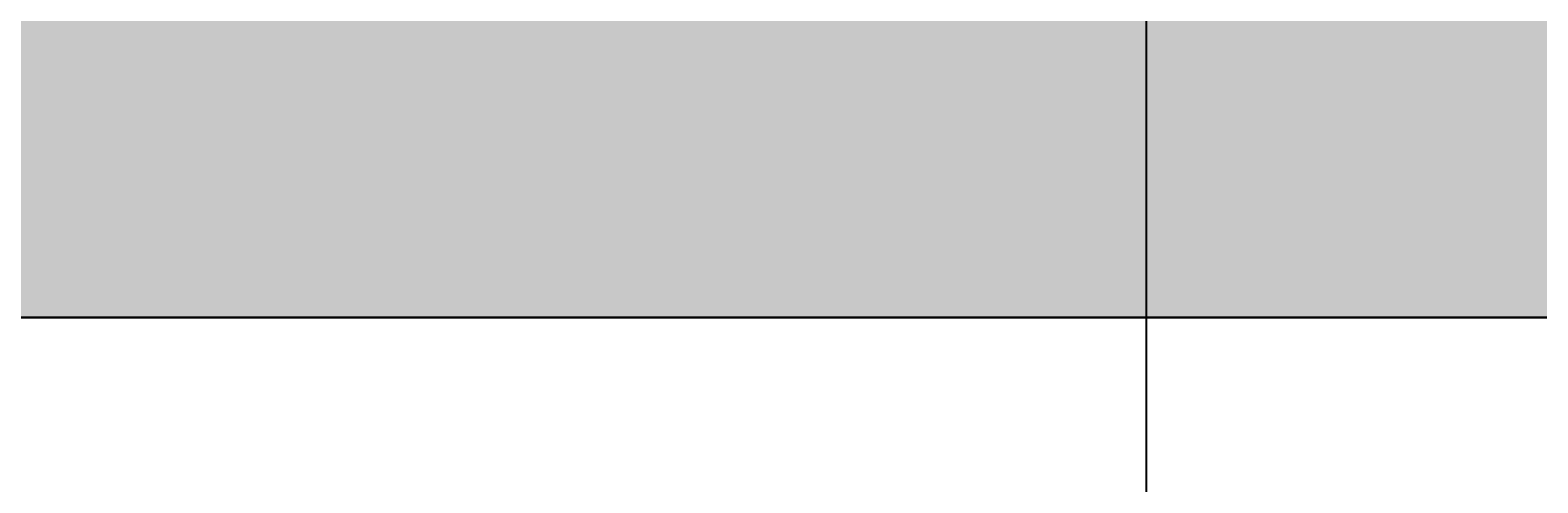
# Model space of a CAD drawing. Units: inches. Extents: x -301 to 715, y -607 to 364.
# Tile 16 of 141: x 18 to 59, y -486 to -474. Entities that reach past the tile are written whole.
import ezdxf

# ---------------------------------------------------------------- set-up
doc = ezdxf.new("R2010")
doc.units = ezdxf.units.IN
doc.header["$MEASUREMENT"] = 0
for name, color, linetype, lineweight in [('A-ANNO-DIMS', 2, 'Continuous', 18), ('A-GRND', 7, 'Continuous', 25), ('A-SECT-PATT', 8, 'Continuous', 13)]:
    doc.layers.add(name, color=color, linetype=linetype, lineweight=lineweight)
doc.styles.get("Standard").update_dxf_attribs({"font": 'arial.ttf'})
doc.dimstyles.get("Standard").update_dxf_attribs({"dimtxt": 0.18, "dimasz": 0.18, "dimexe": 0.18, "dimexo": 0.0625, "dimgap": 0.09, "dimtad": 0, "dimtih": 1, "dimtoh": 1, "dimdec": 1, "dimzin": 0, "dimdsep": 46, "dimlunit": 4, "dimtxsty": 'Standard', "dimcen": 0.09, "dimclrd": 3, "dimclre": 4, "dimclrt": 6, "dimadec": 0, "dimazin": 0, "dimtfac": 1, "dimtdec": 1, "dimtofl": 0, "dimtmove": 0, "dimatfit": 3, "dimfxl": 1, "dimtfill": 2, "dimtfillclr": 51, "dimtolj": 1, "dimtzin": 0, "dimarcsym": 0})

# ---------------------------------------------------------------- blocks, each defined once
blk = doc.blocks.new('*D176')
at = {"layer": 'A-ANNO-DIMS', "color": 4, "lineweight": -2, "transparency": 16777216}
for p, q in [((148.28, -324.477), (215.605, -324.477)), ((-15.22, -540.477), (215.605, -540.477))]:
    blk.add_line(p, q, dxfattribs=at)
at = {"layer": 'A-ANNO-DIMS', "color": 3, "lineweight": -2, "transparency": 16777216}
for p, q in [((215.425, -324.657), (215.425, -432.296)), ((215.425, -540.297), (215.425, -432.659))]:
    blk.add_line(p, q, dxfattribs=at)
at = {"layer": 'A-ANNO-DIMS', "color": 3, "transparency": 16777216}
for points in [[(215.395, -324.657), (215.455, -324.657), (215.425, -324.477)], [(215.395, -540.297), (215.455, -540.297), (215.425, -540.477)]]:
    blk.add_solid(points, dxfattribs=at)
at = {"layer": 'Defpoints', "color": 0, "transparency": 16777216}
for p in [(148.218, -324.477), (-15.282, -540.477), (215.425, -540.477)]:
    blk.add_point(p, dxfattribs=at)
at = {"layer": 'A-ANNO-DIMS', "color": 6, "transparency": 16777216, "insert": (215.425, -432.477), "char_height": 0.18, "attachment_point": 5, "bg_fill": 1, "box_fill_scale": 1.25, "bg_fill_color": 51, "bg_fill_transparency": 0}
blk.add_mtext('\\A1;18\'-0"', dxfattribs=at)
blk = doc.blocks.new('*D181')
at = {"layer": 'A-ANNO-DIMS', "color": 4, "lineweight": -2, "transparency": 16777216}
for p, q in [((48.468, -433.54), (48.468, -573.809)), ((12.718, -463.54), (12.718, -573.809))]:
    blk.add_line(p, q, dxfattribs=at)
at = {"layer": 'A-ANNO-DIMS', "color": 3, "lineweight": -2, "transparency": 16777216}
for p, q in [((12.898, -573.629), (30.264, -573.629)), ((48.288, -573.629), (30.922, -573.629))]:
    blk.add_line(p, q, dxfattribs=at)
at = {"layer": 'A-ANNO-DIMS', "color": 3, "transparency": 16777216}
for points in [[(12.898, -573.599), (12.898, -573.659), (12.718, -573.629)], [(48.288, -573.599), (48.288, -573.659), (48.468, -573.629)]]:
    blk.add_solid(points, dxfattribs=at)
at = {"layer": 'Defpoints', "color": 0, "transparency": 16777216}
for p in [(48.468, -433.477), (12.718, -463.477), (48.468, -573.629)]:
    blk.add_point(p, dxfattribs=at)
at = {"layer": 'A-ANNO-DIMS', "color": 6, "transparency": 16777216, "insert": (30.593, -573.629), "char_height": 0.18, "attachment_point": 5, "bg_fill": 1, "box_fill_scale": 1.25, "bg_fill_color": 51, "bg_fill_transparency": 0}
blk.add_mtext('\\A1;3\'-0"', dxfattribs=at)
blk = doc.blocks.new('*D190')
at = {"layer": 'A-ANNO-DIMS', "color": 4, "lineweight": -2, "transparency": 16777216}
for p, q in [((129.193, -481.477), (-266.112, -481.477)), ((124.193, -511.477), (-266.112, -511.477))]:
    blk.add_line(p, q, dxfattribs=at)
at = {"layer": 'A-ANNO-DIMS', "color": 3, "lineweight": -2, "transparency": 16777216}
for p, q in [((-265.932, -481.657), (-265.932, -496.296)), ((-265.932, -511.297), (-265.932, -496.659))]:
    blk.add_line(p, q, dxfattribs=at)
at = {"layer": 'A-ANNO-DIMS', "color": 3, "transparency": 16777216}
for points in [[(-265.962, -481.657), (-265.902, -481.657), (-265.932, -481.477)], [(-265.962, -511.297), (-265.902, -511.297), (-265.932, -511.477)]]:
    blk.add_solid(points, dxfattribs=at)
at = {"layer": 'Defpoints', "color": 0, "transparency": 16777216}
for p in [(129.255, -481.477), (-265.932, -511.477), (124.255, -511.477)]:
    blk.add_point(p, dxfattribs=at)
at = {"layer": 'A-ANNO-DIMS', "color": 6, "transparency": 16777216, "insert": (-265.932, -496.477), "char_height": 0.18, "attachment_point": 5, "bg_fill": 1, "box_fill_scale": 1.25, "bg_fill_color": 51, "bg_fill_transparency": 0}
blk.add_mtext('\\A1;2\'-6"', dxfattribs=at)
blk = doc.blocks.new('*D191')
at = {"layer": 'A-ANNO-DIMS', "color": 4, "lineweight": -2, "transparency": 16777216}
for p, q in [((129.193, -481.477), (-266.112, -481.477)), ((114.193, -540.477), (-266.112, -540.477))]:
    blk.add_line(p, q, dxfattribs=at)
at = {"layer": 'A-ANNO-DIMS', "color": 3, "lineweight": -2, "transparency": 16777216}
for p, q in [((-265.932, -481.657), (-265.932, -510.797)), ((-265.932, -540.297), (-265.932, -511.158))]:
    blk.add_line(p, q, dxfattribs=at)
at = {"layer": 'A-ANNO-DIMS', "color": 3, "transparency": 16777216}
for points in [[(-265.962, -481.657), (-265.902, -481.657), (-265.932, -481.477)], [(-265.962, -540.297), (-265.902, -540.297), (-265.932, -540.477)]]:
    blk.add_solid(points, dxfattribs=at)
at = {"layer": 'Defpoints', "color": 0, "transparency": 16777216}
for p in [(129.255, -481.477), (-265.932, -540.477), (114.255, -540.477)]:
    blk.add_point(p, dxfattribs=at)
at = {"layer": 'A-ANNO-DIMS', "color": 6, "transparency": 16777216, "insert": (-265.932, -510.977), "char_height": 0.18, "attachment_point": 5, "bg_fill": 1, "box_fill_scale": 1.25, "bg_fill_color": 51, "bg_fill_transparency": 0}
blk.add_mtext('\\A1;4\'-11"', dxfattribs=at)

msp = doc.modelspace()

# ---------------------------------------------------------------- hatches: boundary and pattern name
at = {"layer": 'A-SECT-PATT'}
h = msp.add_hatch(dxfattribs=at)
h.set_pattern_fill('AR-CONC', color=256, scale=0.5)
h.set_pattern_definition([(50, (10.3213, 33.8764), (3.586301, -0.31376), [0.375, -4.125]), (355, (10.3213, 33.8764), (-0.693757, 3.76096), [0.3, -3.3]), (100.45144, (10.62, 33.8502), (2.892544, 3.4472), [0.3187, -3.50571]), (46.1842, (10.3213, 34.8764), (5.336207, -0.827596), [0.5625, -6.1875]), (96.6356, (10.766, 34.8074), (4.67331, 4.870593), [0.47805, -5.25857]), (351.1842, (10.321, 34.8764), (4.67331, 4.870593), [0.45, -4.95]), (21, (10.8213, 34.6264), (2.984535, -2.013094), [0.375, -4.125]), (326, (10.8213, 34.6264), (1.216577, 3.62575), [0.3, -3.3]), (71.45144, (11.07, 34.4586), (4.201112, 1.612656), [0.3187, -3.50571]), (37.5, (10.3213, 33.8764), (0.0607993, 1.6644693), [0, -3.26, 0, -3.35, 0, -3.3125]), (7.5, (10.3213, 33.8764), (1.3153477, 1.9720586), [0, -1.91, 0, -3.185, 0, -1.2625]), (327.5, (9.2063, 33.8764), (2.6691122, -0.1127744), [0, -1.25, 0, -3.9, 0, -5.175]), (317.5, (8.7063, 33.8764), (2.915931, 0.500525), [0, -1.625, 0, -2.59, 0, -3.675])])
h.paths.add_polyline_path([(-56.282, -535.477), (-61.282, -535.477), (-61.282, -540.477), (-15.282, -540.477), (-15.282, -535.477), (-20.282, -535.477)])
h.paths.add_polyline_path([(119.255, -535.477), (114.255, -535.477), (114.255, -540.477), (163.255, -540.477), (163.255, -535.477), (158.255, -535.477)])
h.paths.add_polyline_path([(-206.282, -471.477), (-209.282, -471.477), (-209.282, -481.477), (-206.282, -481.477), (-194.282, -481.477), (-194.282, -471.477)])
h.paths.add_polyline_path([(-41.282, -481.477), (-41.282, -471.477), (-185.282, -471.477), (-185.282, -481.477), (-180.282, -481.477)])
h.paths.add_polyline_path([(134.255, -481.477), (134.255, -471.477), (-35.282, -471.477), (-35.282, -481.477), (-30.282, -481.477)])
h.paths.add_polyline_path([(155.218, -481.477), (158.218, -481.477), (158.218, -471.477), (153.218, -471.477), (143.218, -471.477), (143.218, -481.477), (148.255, -481.477)])
h.paths.add_polyline_path([(-193.88, -356.477), (-193.904, -361.477), (143.218, -361.477), (143.218, -356.477)])

# ---------------------------------------------------------------- linework, layer by layer
at = {"layer": 'A-GRND'}
msp.add_line((-206.282, -481.477), (155.218, -481.477), dxfattribs=at)

# ---------------------------------------------------------------- dimensions: what is measured, and where the dimension line sits
at = {"layer": 'A-ANNO-DIMS'}
for base, p1, p2, picture, middle in [((215.425, -540.477), (148.218, -324.477), (-15.282, -540.477), '*D176', (215.425, -432.477)), ((-265.932, -540.477), (129.255, -481.477), (114.255, -540.477), '*D191', (-265.932, -510.977)), ((-265.932, -511.477), (129.255, -481.477), (124.255, -511.477), '*D190', (-265.932, -496.477))]:
    dim = msp.add_linear_dim(base=base, p1=p1, p2=p2, angle=90, dimstyle='Standard', override={"dimdec": 1, "dimlfac": 1, "dimrnd": 0, "dimzin": 1, "dimdsep": 46, "dimlunit": 4, "dimfrac": 2}, dxfattribs=at)
    dim.commit()
    dim.dimension.update_dxf_attribs({"geometry": picture, "text_midpoint": middle})
dim = msp.add_linear_dim(base=(48.467984, -573.628877), p1=(12.717984, -463.47741), p2=(48.467984, -433.47741), dimstyle='Standard', override={"dimdec": 1, "dimlfac": 1, "dimrnd": 0, "dimzin": 1, "dimdsep": 46, "dimlunit": 4, "dimfrac": 2}, dxfattribs=at)
dim.commit()
dim.dimension.update_dxf_attribs({"geometry": '*D181', "text_midpoint": (30.592984, -573.628877)})

doc.saveas('drawing.dxf')
